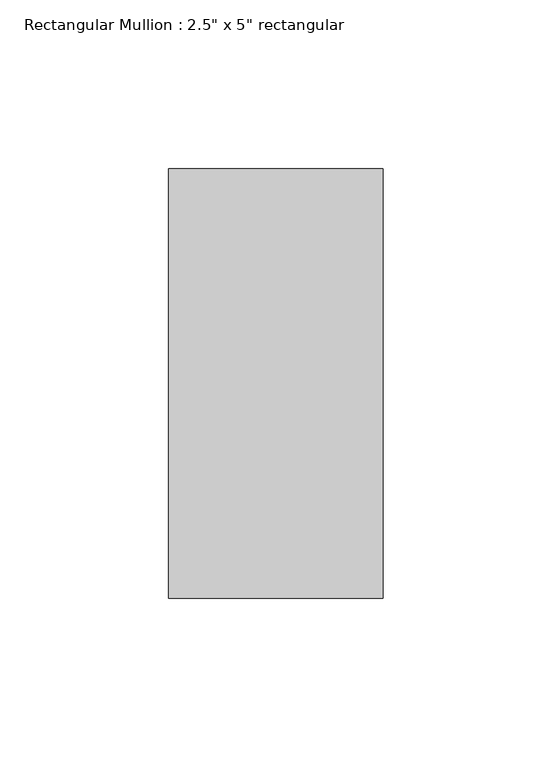
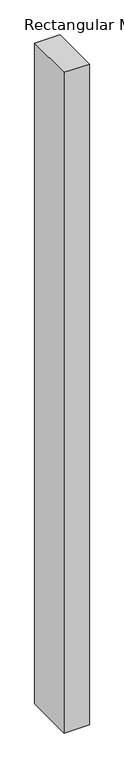
"""IFC4 building model written with IfcOpenShell, lengths in millimetres: member geometry."""

from ifc_helpers import new_model, si_unit, frame, origin, place, context, project, spatial, polyline, outline, extrude, source, transform, mapped, element, save


def member_334bbce8(model_context):
    return source(origin(), model_context, "Body", "SweptSolid", [
        extrude(outline(polyline([(31.75, 63.5), (31.75, -63.5), (-31.75, -63.5), (-31.75, 63.5), (31.75, 63.5)])), frame((0.0, 0.0, -1748.0218004), z_axis=(0.0, 0.0, 1.0), x_axis=(1.0, 0.0, 0.0)), (0.0, 0.0, 1.0), 1748.0218004),
    ])


if __name__ == "__main__":
    model = new_model("IFC4")
    model_context = context("Model", 3, world=origin())
    ifc_project = project(units=[si_unit("LENGTHUNIT", "METRE", prefix="MILLI")], contexts=[model_context])
    site = spatial("IfcSite", under=ifc_project)
    building = spatial("IfcBuilding", under=site)
    placement = place(None, origin())
    member_shape = member_334bbce8(model_context)
    element("IfcMember", 1, ObjectType="Rectangular Mullion : 2.5\" x 5\" rectangular", at=placement, inside=building, context=model_context, shape_type="MappedRepresentation", body=[
        mapped(member_shape, transform((0.0, 0.0, 0.0), x_axis=(1.0, 0.0, 0.0), y_axis=(0.0, 1.0, 0.0), z_axis=(0.0, 0.0, 1.0))),
    ])
    save(model, "model.ifc")

# Revit data of these elements
# Type "Rectangular Mullion : 2.5\" x 5\" rectangular"
#   built-in parameter 1007304 = 0.416667 (stored number, unit not read)
#   built-in parameter 1007301 = 0.104167 (stored number, unit not read)
#   built-in parameter 1007300 = 0.104167 (stored number, unit not read)
# Element 1 (IfcMember, "Rectangular Mullion : 2.5\" x 5\" rectangular")
#   Materials on its faces: "Aluminum"
# Materials
#   "Aluminum": class "Metal", colour RGB 247 247 247, transparency 0, Description = "Aluminum 6061", Cost = 0
